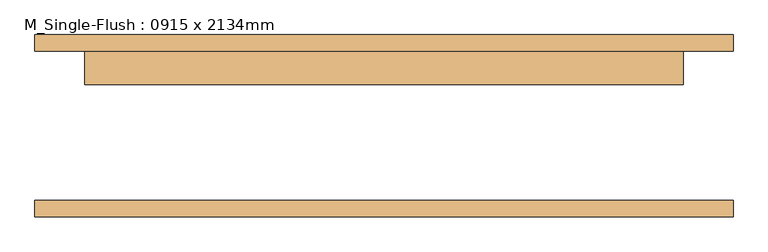
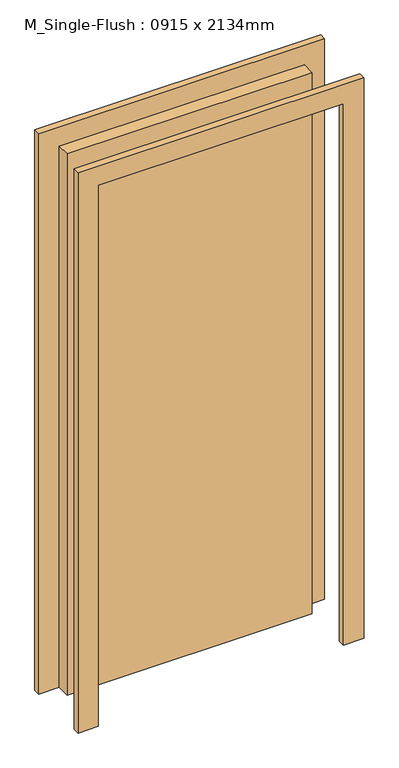
"""IFC4 building model written with IfcOpenShell, lengths in millimetres: door geometry, M_Single-Flush : 0915 x 2134mm."""

from ifc_helpers import new_model, si_unit, frame, origin, origin_with_axes, place, context, project, spatial, polyline, outline, extrude, source, transform, mapped, element, save


def m_single_flush_0915_x_2134mm_1ddf3370(model_context):
    return source(origin(), model_context, "Body", "SweptSolid", [
        extrude(outline(polyline([(2210.0, -533.5), (0.0, -533.5), (0.0, -457.5), (2134.0, -457.5), (2134.0, 457.5), (0.0, 457.5), (0.0, 533.5), (2210.0, 533.5), (2210.0, -533.5)])), frame((0.0, 114.3, 0.0), z_axis=(0.0, 1.0, 0.0), x_axis=(0.0, 0.0, 1.0)), (0.0, 0.0, 1.0), 25.0),
        extrude(outline(polyline([(2210.0, 533.5), (2210.0, -533.5), (0.0, -533.5), (0.0, -457.5), (2134.0, -457.5), (2134.0, 457.5), (0.0, 457.5), (0.0, 533.5), (2210.0, 533.5)])), frame((0.0, -139.3, 0.0), z_axis=(0.0, 1.0, 0.0), x_axis=(0.0, 0.0, 1.0)), (0.0, 0.0, 1.0), 25.0),
        extrude(outline(polyline([(457.5, 63.3), (-457.5, 63.3), (-457.5, 114.3), (457.5, 114.3), (457.5, 63.3)])), origin_with_axes(), (0.0, 0.0, 1.0), 2134.0),
    ])


if __name__ == "__main__":
    model = new_model("IFC4")
    model_context = context("Model", 3, world=origin())
    ifc_project = project(units=[si_unit("LENGTHUNIT", "METRE", prefix="MILLI")], contexts=[model_context])
    site = spatial("IfcSite", under=ifc_project)
    building = spatial("IfcBuilding", under=site)
    placement = place(None, origin())
    m_single_flush_0915_x_2134mm_shape = m_single_flush_0915_x_2134mm_1ddf3370(model_context)
    element("IfcDoor", 1, ObjectType="M_Single-Flush : 0915 x 2134mm", at=placement, inside=building, context=model_context, shape_type="MappedRepresentation", body=[
        mapped(m_single_flush_0915_x_2134mm_shape, transform((0.0, 0.0, 0.0), x_axis=(1.0, 0.0, 0.0), y_axis=(0.0, 1.0, 0.0), z_axis=(0.0, 0.0, 1.0))),
    ])
    save(model, "model.ifc")

# Revit data of these elements
# Type "M_Single-Flush : 0915 x 2134mm"
#   Type Mark = "20"
#   Construction Type Id = "MDOOR"
#   Analytic Construction = "Metal"
#   Thickness = 0.167323 ft
#   Thermal Resistance (R) = 0.270117 (m²·K)/W
#   Heat Transfer Coefficient (U) = 3.7021 W/(m²·K)
#   Height = 7.001312 ft
#   Trim Projection Ext = 0.082021 ft
#   Trim Projection Int = 0.082021 ft
#   Trim Width = 0.249344 ft
#   Width = 3.001969 ft
#   Define Thermal Properties by = 1
#   Define Thermal Properties by = 1
#   Door Material = Door - Panel
#   Frame Material = Door - Frame
#   Visual Light Transmittance = 0
#   Solar Heat Gain Coefficient = 0
#   Function = (empty or 0)
#   Wall Closure = (empty or 0)
# Element 1 (IfcDoor, "M_Single-Flush : 0915 x 2134mm")
#   Materials on its faces: "Door - Frame", "Door - Panel"
# Materials
#   "Door - Panel": class "Wood", colour RGB 210 159 95, transparency 0, Cost = 0
#   "Door - Frame": colour RGB 118 70 51, transparency 0, Cost = 0
